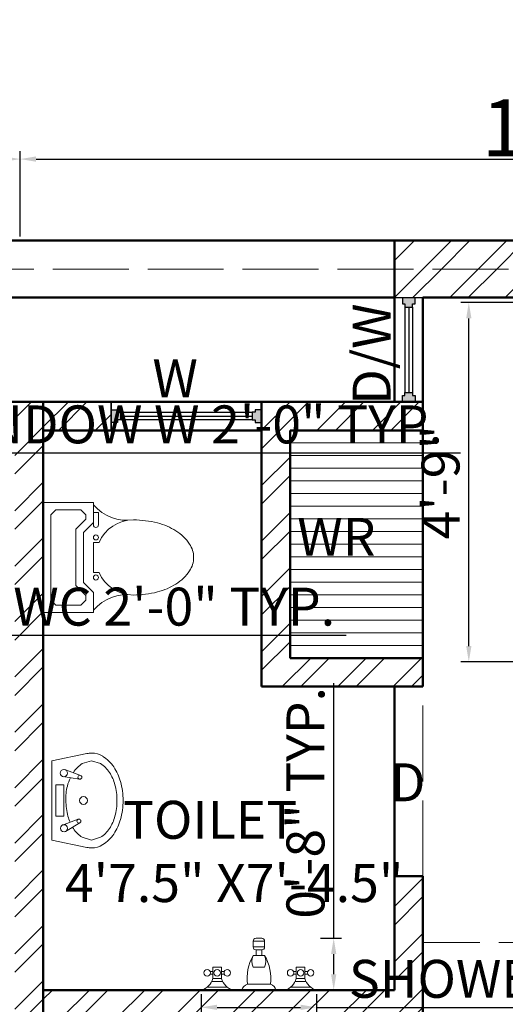
# Model space of a CAD drawing. Units: millimetres. Extents: x 4237 to 5109, y 21391 to 22486.
# Tile 11 of 17: x 4458 to 4535, y 22320 to 22476. Entities that reach past the tile are written whole.
import ezdxf

# ---------------------------------------------------------------- set-up
doc = ezdxf.new("R2010")
doc.units = ezdxf.units.MM
doc.linetypes.add('ACAD_ISO02W100', pattern=[15, 12, -3])
for name, color, linetype, lineweight in [('A-ANNO-DIMS', 2, 'Continuous', 18), ('A-ANNO-TEXT', 7, 'Continuous', 18), ('A-AREA-IDEN', 3, 'Continuous', 18), ('A-FLOR-OVHD', 1, 'ACAD_ISO02W100', 18), ('A-FURN', 8, 'Continuous', 18), ('A-FURN-CASE', 31, 'Continuous', 13), ('A-WALL', 7, 'Continuous', 50), ('A-WALL-PATT', 252, 'Continuous', 13), ('windows', 140, 'Continuous', 25)]:
    doc.layers.add(name, color=color, linetype=linetype, lineweight=lineweight)
doc.styles.get("Standard").update_dxf_attribs({"font": 'arial.ttf'})
doc.dimstyles.new('ISO-25', dxfattribs={"dimtxt": 6, "dimasz": 2.5, "dimexe": 1.25, "dimexo": 0.625, "dimtad": 1, "dimdec": 1, "dimlunit": 4, "dimtxsty": 'Standard', "dimcen": 2.5, "dimadec": 0, "dimazin": 0, "dimtfac": 1, "dimtdec": 1, "dimtmove": 0, "dimatfit": 3, "dimfxl": 1, "dimarcsym": 0})

# ---------------------------------------------------------------- blocks, each defined once
blk = doc.blocks.new('A$C5EF6120A')
at = {"linetype": 'ByBlock'}
for p, q in [((0, 0.762), (0, 0.508)), ((0, 0.762), (0.5588, 0.762)), ((0.5588, 0.762), (0.5588, 0.508)), ((0.0381, 0.6985), (0.0635, 0.7239)), ((0.0635, 0.7239), (0.4953, 0.7239)), ((0.4953, 0.7239), (0.5207, 0.6985)), ((0.0381, 0.6985), (0.0381, 0.5715)), ((0.5207, 0.6985), (0.5207, 0.5715)), ((0.0635, 0.5461), (0.0381, 0.5715)), ((0.1366, 0.5969), (0.0858, 0.5461)), ((0.1524, 0.5588), (0.1016, 0.508)), ((0.1366, 0.5969), (0.4222, 0.5969)), ((0.1524, 0.5588), (0.4064, 0.5588)), ((0.4064, 0.5588), (0.4572, 0.508)), ((0.4222, 0.5969), (0.473, 0.5461)), ((0.5207, 0.5715), (0.4953, 0.5461)), ((0, 0.508), (0.1016, 0.508)), ((0.0508, 0.508), (0.0508, 0.4826)), ((0.0635, 0.5461), (0.0858, 0.5461)), ((0.1143, 0.508), (0.1016, 0.508)), ((0.2032, 0.508), (0.2032, 0.4794)), ((0.3556, 0.508), (0.2032, 0.508)), ((0.3556, 0.508), (0.3556, 0.4794)), ((0.5588, 0.508), (0.4572, 0.508)), ((0.4953, 0.5461), (0.473, 0.5461)), ((0.0508, 0.4826), (0.1143, 0.4826))]:
    blk.add_line(p, q, dxfattribs=at)
blk.add_lwpolyline([(0.0889, 0.3048, 0.063415), (0.1044, 0.183, 0.076468), (0.1447, 0.0893, 0.107136), (0.2118, 0.0204, 0.147373), (0.2794, 0, 0.147373), (0.347, 0.0204, 0.107136), (0.4141, 0.0893, 0.076468), (0.4544, 0.183, 0.063415), (0.4699, 0.3048, 0.063415)], format="xyb", dxfattribs=at)
for centre in [(0.1778, 0.4953), (0.381, 0.4953)]:
    blk.add_circle(centre, 0.0127, dxfattribs=at)
for centre, radius, start, end in [((-0.1375, 0.3358), 0.2285, 352.2011, 48.911), ((0.1143, 0.4953), 0.0127, 270, 90), ((0.6963, 0.3358), 0.2285, 131.089, 187.7989), ((0.2794, 0.3048), 0.1905, 113.5782, 180), ((0.2794, 0.3048), 0.1905, 0, 66.4218)]:
    blk.add_arc(centre, radius, start, end, dxfattribs=at)
blk = doc.blocks.new('A$C60F95712')
for p, q in [((0.05, 0.45), (0.003, 0.2283)), ((0.55, 0.45), (0.05, 0.45)), ((0.597, 0.2283), (0.55, 0.45)), ((0.1448, 0.3831), (0.1814, 0.2836)), ((0.4, 0.425), (0.2, 0.425)), ((0.2, 0.425), (0.2, 0.375)), ((0.2, 0.375), (0.4, 0.375)), ((0.4, 0.375), (0.4, 0.425)), ((0.4514, 0.3804), (0.4348, 0.2751)), ((0.1035, 0.3639), (0.1588, 0.2727)), ((0.4953, 0.3684), (0.459, 0.2688))]:
    blk.add_line(p, q)
for points in [[(0.1307, 0.319, 0.008163), (0.1232, 0.3143, 0.107176), (0.0669, 0.2578), (0.05, 0.2), (0.0669, 0.1422, 0.107176), (0.1232, 0.0857, 0.078233), (0.2003, 0.0515, 0.065516), (0.3, 0.0383, 0.065516), (0.3997, 0.0515, 0.078233), (0.4768, 0.0857, 0.107176), (0.5331, 0.1422), (0.55, 0.2)], [(0.4439, 0.3328, 0.046779), (0.3911, 0.3524, 0.080145), (0.3, 0.3617, 0.065516), (0.2003, 0.3485, 0.037125), (0.1623, 0.3353, 0.107176)], [(0.55, 0.2), (0.5331, 0.2578, 0.107176), (0.4768, 0.3143, 0.000976), (0.4758, 0.3149, 0.080145)]]:
    blk.add_lwpolyline(points, format="xyb")
for centre, radius in [((0.1241, 0.3735), 0.0228), ((0.4733, 0.3744), 0.0228), ((0.1696, 0.2793), 0.0126), ((0.3, 0.25), 0.025), ((0.4472, 0.2731), 0.0126)]:
    blk.add_circle(centre, radius)
for centre, radius, start, end in [((0.1362, 0.2), 0.1362, 168.02396, 180), ((0.1362, 0.2), 0.1362, 180, 211.85353), ((0.4638, 0.2), 0.1362, 328.14647, 0), ((0.4638, 0.2), 0.1362, 0, 11.97604), ((0.2147, 0.2488), 0.2286, 211.85353, 236.30993), ((0.3853, 0.2488), 0.2286, 303.69007, 328.14647), ((0.2662, 0.3261), 0.3215, 236.30993, 254.56292), ((0.3, 0.4484), 0.4484, 254.56292, 270), ((0.3, 0.4484), 0.4484, 270, 285.43708), ((0.3338, 0.3261), 0.3215, 285.43708, 303.69007)]:
    blk.add_arc(centre, radius, start, end)
blk = doc.blocks.new('Faucet - Bathroom front')
for p, q in [((-0.5, 4.25), (0.5, 4.25)), ((0.5, 3.75), (-0.5, 3.75)), ((-0.25, 3), (-0.25, 3.5)), ((0.25, 3.5), (0.25, 3)), ((-0.5, 3), (0.5, 3)), ((0.5, 2), (-0.5, 2)), ((-4, 1.625), (-4.25, 1.625)), ((-4, 1.375), (-4.25, 1.375)), ((-3.25, 1.625), (-3, 1.625)), ((-3.25, 1.375), (-3, 1.375)), ((3.25, 1.625), (3, 1.625)), ((3.25, 1.375), (3, 1.375)), ((4, 1.625), (4.25, 1.625)), ((4, 1.375), (4.25, 1.375)), ((-5, 0), (-2.25, 0)), ((-4.5087, 0.25), (-2.7408, 0.25)), ((-3.1442, 0.75), (-4.0979, 0.75)), ((-1.5, 0), (1.5, 0)), ((-1, 0.5), (1, 0.5)), ((2.25, 0), (5, 0)), ((2.7413, 0.25), (4.5092, 0.25)), ((4.1058, 0.75), (3.1521, 0.75))]:
    blk.add_line(p, q)
for points in [[(-0.25, 4.5), (0.25, 4.5)], [(-0.5, 3.75), (-0.5, 4.25)], [(0.25, 3.5), (-0.25, 3.5)], [(0.5, 4.25), (0.5, 3.75)]]:
    blk.add_lwpolyline(points)
for points in [[(-4, 1), (-4, 2), (-3.25, 2), (-3.25, 1)], [(3.25, 1), (3.25, 2), (4, 2), (4, 1)]]:
    blk.add_lwpolyline(points, close=True)
for centre in [(-4.5, 1.5), (-3.625, 1.5), (-2.75, 1.5), (2.75, 1.5), (3.625, 1.5), (4.5, 1.5)]:
    blk.add_circle(centre, 0.2795)
for centre, radius, start, end in [((-0.2575, 4.2575), 0.2426, 88.22243, 181.7776), ((0.2575, 4.2575), 0.2426, 358.2224, 91.77757), ((-0.2575, 3.7425), 0.2426, 178.2224, 271.7776), ((0.2575, 3.7425), 0.2426, 268.2224, 1.777565), ((3, 1), 4.0311, 150.2551, 187.125), ((0.6413, 2.5), 1.246, 156.3417, 203.6583), ((-3, 1), 4.0311, 352.875, 29.74488), ((-0.6413, 2.5), 1.246, 336.3417, 23.65835), ((-5.375, 1.375), 1.4252, 285.2551, 344.7449), ((-1.875, 1.375), 1.4252, 195.2551, 254.7449), ((1.875, 1.375), 1.4252, 285.2551, 344.7449), ((5.375, 1.375), 1.4252, 195.2551, 254.7449), ((-0.7962, -0.2038), 0.7327, 106.1502, 163.8498), ((0.7962, -0.2038), 0.7327, 16.1502, 73.84979)]:
    blk.add_arc(centre, radius, start, end)
blk = doc.blocks.new('*D56')
at = {"layer": 'A-ANNO-DIMS', "color": 0, "lineweight": -2, "transparency": 16777216}
for p, q in [((4271.65, 22441.33), (4271.65, 22454.84)), ((4274.15, 22453.59), (4455.8, 22453.59)), ((4458.3, 22441.33), (4458.3, 22454.84))]:
    blk.add_line(p, q, dxfattribs=at)
at = {"layer": 'A-ANNO-DIMS', "color": 0, "transparency": 16777216}
for points in [[(4274.15, 22454.01), (4274.15, 22453.17), (4271.65, 22453.59)], [(4455.8, 22454.01), (4455.8, 22453.17), (4458.3, 22453.59)]]:
    blk.add_solid(points, dxfattribs=at)
at = {"layer": 'Defpoints', "color": 0, "transparency": 16777216}
for p in [(4458.3, 22453.59), (4271.65, 22440.7), (4458.3, 22440.7)]:
    blk.add_point(p, dxfattribs=at)
at = {"layer": 'A-ANNO-DIMS', "color": 0, "transparency": 16777216, "insert": (4364.98, 22464.83), "char_height": 9, "attachment_point": 5}
blk.add_mtext('15\'-6{\\H1x;\\S1/2;}"', dxfattribs=at)
blk = doc.blocks.new('*D57')
at = {"layer": 'A-ANNO-DIMS', "color": 0, "lineweight": -2, "transparency": 16777216}
for p, q in [((4458.3, 22441.33), (4458.3, 22454.84)), ((4460.8, 22453.59), (4642.45, 22453.59)), ((4644.95, 22441.33), (4644.95, 22454.84))]:
    blk.add_line(p, q, dxfattribs=at)
at = {"layer": 'A-ANNO-DIMS', "color": 0, "transparency": 16777216}
for points in [[(4460.8, 22454.01), (4460.8, 22453.17), (4458.3, 22453.59)], [(4642.45, 22454.01), (4642.45, 22453.17), (4644.95, 22453.59)]]:
    blk.add_solid(points, dxfattribs=at)
at = {"layer": 'Defpoints', "color": 0, "transparency": 16777216}
for p in [(4644.95, 22453.59), (4458.3, 22440.7), (4644.95, 22440.7)]:
    blk.add_point(p, dxfattribs=at)
at = {"layer": 'A-ANNO-DIMS', "color": 0, "transparency": 16777216, "insert": (4551.63, 22464.83), "char_height": 9, "attachment_point": 5}
blk.add_mtext('15\'-6{\\H1x;\\S1/2;}"', dxfattribs=at)
blk = doc.blocks.new('WIN-A')
blk.add_line((0, 4.5), (0, 0))
blk.add_lwpolyline([(0, 4.5), (23.8, 4.5), (23.8, 0), (0, 0)], close=True)
blk = doc.blocks.new('*D67')
at = {"layer": 'A-ANNO-DIMS', "color": 0, "lineweight": -2, "transparency": 16777216}
for p, q in [((4540.51, 22430.91), (4527.94, 22430.91)), ((4529.19, 22376.6), (4529.19, 22428.41)), ((4540.51, 22374.1), (4527.94, 22374.1))]:
    blk.add_line(p, q, dxfattribs=at)
at = {"layer": 'A-ANNO-DIMS', "color": 0, "transparency": 16777216}
for points in [[(4528.78, 22428.41), (4529.61, 22428.41), (4529.19, 22430.91)], [(4528.78, 22376.6), (4529.61, 22376.6), (4529.19, 22374.1)]]:
    blk.add_solid(points, dxfattribs=at)
at = {"layer": 'Defpoints', "color": 0, "transparency": 16777216}
for p in [(4529.19, 22430.91), (4541.13, 22430.91), (4541.13, 22374.1)]:
    blk.add_point(p, dxfattribs=at)
at = {"layer": 'A-ANNO-DIMS', "color": 0, "transparency": 16777216, "insert": (4525.5, 22402.5), "char_height": 6, "attachment_point": 5, "rotation": 90}
blk.add_mtext('4\'-9"', dxfattribs=at)
blk = doc.blocks.new('*D76')
at = {"layer": 'A-ANNO-DIMS', "color": 0, "lineweight": -2, "transparency": 16777216}
for p, q in [((4429.2, 22381.26), (4429.2, 22377.08)), ((4452.95, 22381.26), (4452.95, 22377.08)), ((4431.7, 22378.33), (4450.45, 22378.33)), ((4452.95, 22378.33), (4509.81, 22378.33))]:
    blk.add_line(p, q, dxfattribs=at)
at = {"layer": 'A-ANNO-DIMS', "color": 0, "transparency": 16777216}
for points in [[(4431.7, 22378.74), (4431.7, 22377.91), (4429.2, 22378.33)], [(4450.45, 22378.74), (4450.45, 22377.91), (4452.95, 22378.33)]]:
    blk.add_solid(points, dxfattribs=at)
at = {"layer": 'Defpoints', "color": 0, "transparency": 16777216}
for p in [(4429.2, 22381.89), (4452.95, 22381.89), (4452.95, 22378.33)]:
    blk.add_point(p, dxfattribs=at)
at = {"layer": 'A-ANNO-DIMS', "color": 0, "transparency": 16777216, "insert": (4482.63, 22382.05), "char_height": 6, "attachment_point": 5}
blk.add_mtext('WC 2\'-0" TYP.', dxfattribs=at)
blk = doc.blocks.new('*D80')
at = {"layer": 'A-ANNO-DIMS', "color": 0, "lineweight": -2, "transparency": 16777216}
for p, q in [((4414.15, 22410.08), (4414.15, 22405.88)), ((4437.95, 22410.08), (4437.95, 22405.88)), ((4416.65, 22407.13), (4435.45, 22407.13)), ((4437.95, 22407.13), (4527.87, 22407.13))]:
    blk.add_line(p, q, dxfattribs=at)
at = {"layer": 'A-ANNO-DIMS', "color": 0, "transparency": 16777216}
for points in [[(4416.65, 22407.55), (4416.65, 22406.71), (4414.15, 22407.13)], [(4435.45, 22407.55), (4435.45, 22406.71), (4437.95, 22407.13)]]:
    blk.add_solid(points, dxfattribs=at)
at = {"layer": 'Defpoints', "color": 0, "transparency": 16777216}
for p in [(4414.15, 22410.7), (4437.95, 22410.7), (4437.95, 22407.13)]:
    blk.add_point(p, dxfattribs=at)
at = {"layer": 'A-ANNO-DIMS', "color": 0, "transparency": 16777216, "insert": (4484.16, 22410.86), "char_height": 6, "attachment_point": 5}
blk.add_mtext('WINDOW W 2\'-0" TYP.', dxfattribs=at)
blk = doc.blocks.new('*D90')
at = {"layer": 'A-ANNO-DIMS', "color": 0, "lineweight": -2, "transparency": 16777216}
for p, q in [((4486.92, 22321.58), (4486.92, 22318.22)), ((4505.11, 22321.58), (4505.11, 22318.22)), ((4489.42, 22319.47), (4502.61, 22319.47)), ((4505.11, 22319.47), (4585.45, 22319.47))]:
    blk.add_line(p, q, dxfattribs=at)
at = {"layer": 'A-ANNO-DIMS', "color": 0, "transparency": 16777216}
for points in [[(4489.42, 22319.89), (4489.42, 22319.06), (4486.92, 22319.47)], [(4502.61, 22319.89), (4502.61, 22319.06), (4505.11, 22319.47)]]:
    blk.add_solid(points, dxfattribs=at)
at = {"layer": 'Defpoints', "color": 0, "transparency": 16777216}
for p in [(4486.92, 22322.2), (4505.11, 22322.2), (4505.11, 22319.47)]:
    blk.add_point(p, dxfattribs=at)
at = {"layer": 'A-ANNO-DIMS', "color": 0, "transparency": 16777216, "insert": (4546.53, 22323.2), "char_height": 6, "attachment_point": 5}
blk.add_mtext('SHOWER 1\'-6" TYP.', dxfattribs=at)
blk = doc.blocks.new('*D91')
at = {"layer": 'A-ANNO-DIMS', "color": 0, "lineweight": -2, "transparency": 16777216}
for p, q in [((4507.84, 22330.39), (4507.84, 22370.71)), ((4505.74, 22330.39), (4509.09, 22330.39)), ((4507.84, 22324.7), (4507.84, 22327.89)), ((4505.74, 22322.2), (4509.09, 22322.2))]:
    blk.add_line(p, q, dxfattribs=at)
at = {"layer": 'A-ANNO-DIMS', "color": 0, "transparency": 16777216}
for points in [[(4507.42, 22327.89), (4508.26, 22327.89), (4507.84, 22330.39)], [(4507.42, 22324.7), (4508.26, 22324.7), (4507.84, 22322.2)]]:
    blk.add_solid(points, dxfattribs=at)
at = {"layer": 'Defpoints', "color": 0, "transparency": 16777216}
for p in [(4505.11, 22330.39), (4507.84, 22330.39), (4505.11, 22322.2)]:
    blk.add_point(p, dxfattribs=at)
at = {"layer": 'A-ANNO-DIMS', "color": 0, "transparency": 16777216, "insert": (4504.15, 22351.8), "char_height": 6, "attachment_point": 5, "rotation": 90}
blk.add_mtext('0\'-8" TYP.', dxfattribs=at)

msp = doc.modelspace()

# ---------------------------------------------------------------- hatches: boundary and pattern name
at = {"layer": 'A-WALL-PATT'}
h = msp.add_hatch(dxfattribs=at)
h.set_pattern_fill('ANSI32', color=256, scale=0.65)
h.paths.add_polyline_path([(4644.95, 22440.7), (4517.45, 22440.7), (4517.45, 22436.2), (4622.45, 22436.2), (4640.45, 22436.2), (4640.45, 22427.2), (4640.45, 22233.7), (4644.95, 22233.7)])
h = msp.add_hatch(dxfattribs=at)
h.set_pattern_fill('ANSI32', color=256, scale=0.65)
h.paths.add_polyline_path([(4622.45, 22436.2), (4517.45, 22436.2), (4517.45, 22431.7), (4521.95, 22431.7), (4622.45, 22431.7)], flags=17)
h = msp.add_hatch(color=256, dxfattribs=at)
h.dxf.hatch_style = 1
h.paths.add_polyline_path([(4520.7, 22431.7), (4518.7, 22431.7), (4518.7, 22430.7), (4519.09, 22430.7), (4519.09, 22430.19), (4520.31, 22430.19), (4520.31, 22430.7), (4520.7, 22430.7)])
h = msp.add_hatch(color=256, dxfattribs=at)
h.dxf.hatch_style = 1
h.paths.add_polyline_path([(4520.7, 22416.2), (4520.31, 22416.2), (4520.31, 22416.71), (4519.09, 22416.71), (4519.09, 22416.2), (4518.7, 22416.2), (4518.7, 22415.2), (4520.7, 22415.2)])
h = msp.add_hatch(dxfattribs=at)
h.set_pattern_fill('ANSI32', color=256, scale=0.65)
h.paths.add_polyline_path([(4461.95, 22415.2), (4457.45, 22415.2), (4457.45, 22233.7), (4461.95, 22233.7)])
h = msp.add_hatch(dxfattribs=at)
h.set_pattern_fill('ANSI32', color=256, scale=0.65)
h.paths.add_polyline_path([(4472.65, 22415.2), (4461.95, 22415.2), (4461.95, 22410.7), (4472.65, 22410.7)])
h = msp.add_hatch(dxfattribs=at)
h.set_pattern_fill('ANSI32', color=256, scale=0.65)
h.paths.add_polyline_path([(4521.95, 22415.2), (4517.45, 22415.2), (4496.45, 22415.2), (4496.45, 22410.7), (4496.45, 22370.2), (4521.95, 22370.2), (4521.95, 22374.7), (4500.95, 22374.7), (4500.95, 22410.7), (4521.95, 22410.7)])
h = msp.add_hatch(color=256, dxfattribs=at)
h.dxf.hatch_style = 1
h.paths.add_polyline_path([(4474.17, 22413.56), (4473.65, 22413.56), (4473.65, 22413.95), (4472.65, 22413.95), (4472.65, 22411.95), (4473.65, 22411.95), (4473.65, 22412.34), (4474.17, 22412.34)])
h = msp.add_hatch(color=256, dxfattribs=at)
h.dxf.hatch_style = 1
h.paths.add_polyline_path([(4496.45, 22413.95), (4495.45, 22413.95), (4495.45, 22413.56), (4494.94, 22413.56), (4494.94, 22412.34), (4495.45, 22412.34), (4495.45, 22411.95), (4496.45, 22411.95)])
h = msp.add_hatch(dxfattribs=at)
h.set_pattern_fill('ANSI32', color=256, scale=0.65)
h.paths.add_polyline_path([(4521.95, 22340.2), (4517.45, 22340.2), (4517.45, 22322.2), (4461.95, 22322.2), (4461.95, 22317.7), (4521.95, 22317.7)])

# ---------------------------------------------------------------- linework, layer by layer
at = {"layer": 'A-FLOR-OVHD'}
for p, q in [((4521.95, 22340.2), (4521.95, 22370.2)), ((4560.95, 22329.7), (4521.95, 22329.7))]:
    msp.add_line(p, q, dxfattribs=at)
msp.add_lwpolyline([(4640.45, 22032.7), (4640.45, 22436.2), (4276.15, 22436.2), (4276.15, 22032.7)], dxfattribs=at)
at = {"layer": 'A-FURN-CASE'}
for p, q in [((4500.95, 22408.7), (4521.95, 22408.7)), ((4500.95, 22406.7), (4521.95, 22406.7)), ((4500.95, 22404.7), (4521.95, 22404.7)), ((4500.95, 22402.7), (4521.95, 22402.7)), ((4500.95, 22400.7), (4521.95, 22400.7)), ((4500.95, 22398.7), (4521.95, 22398.7)), ((4500.95, 22396.7), (4521.95, 22396.7)), ((4500.95, 22394.7), (4521.95, 22394.7)), ((4500.95, 22392.7), (4521.95, 22392.7)), ((4500.95, 22390.7), (4521.95, 22390.7)), ((4500.95, 22388.7), (4521.95, 22388.7)), ((4500.95, 22386.7), (4521.95, 22386.7)), ((4500.95, 22384.7), (4521.95, 22384.7)), ((4500.95, 22382.7), (4521.95, 22382.7)), ((4500.95, 22380.7), (4521.95, 22380.7)), ((4500.95, 22378.7), (4521.95, 22378.7)), ((4500.95, 22376.7), (4521.95, 22376.7))]:
    msp.add_line(p, q, dxfattribs=at)
at = {"layer": 'A-WALL'}
for p, q in [((4271.65, 22440.7), (4644.95, 22440.7)), ((4517.45, 22440.7), (4517.45, 22415.2)), ((4399.15, 22431.7), (4517.45, 22431.7)), ((4521.95, 22431.7), (4521.95, 22370.2)), ((4521.95, 22431.7), (4622.45, 22431.7)), ((4394.65, 22415.2), (4521.95, 22415.2)), ((4461.95, 22415.2), (4461.95, 22233.7)), ((4496.45, 22415.2), (4496.45, 22370.2)), ((4496.45, 22415.2), (4496.45, 22410.7)), ((4461.95, 22410.7), (4496.45, 22410.7)), ((4500.95, 22410.7), (4500.95, 22374.7)), ((4500.95, 22410.7), (4521.95, 22410.7)), ((4500.95, 22374.7), (4521.95, 22374.7)), ((4496.45, 22370.2), (4521.95, 22370.2)), ((4517.45, 22340.2), (4517.45, 22370.2)), ((4517.45, 22340.2), (4517.45, 22322.2)), ((4517.45, 22340.2), (4521.95, 22340.2)), ((4521.95, 22340.2), (4521.95, 22317.7)), ((4461.95, 22322.2), (4517.45, 22322.2))]:
    msp.add_line(p, q, dxfattribs=at)
at = {"layer": 'windows'}
for p, q in [((4519.09, 22430.19), (4519.09, 22416.71)), ((4519.7, 22430.19), (4519.7, 22416.71)), ((4520.31, 22430.19), (4520.31, 22416.71)), ((4474.17, 22413.56), (4494.94, 22413.56)), ((4474.17, 22412.95), (4494.94, 22412.95)), ((4494.94, 22412.34), (4474.17, 22412.34))]:
    msp.add_line(p, q, dxfattribs=at)
msp.add_lwpolyline([(4517.45, 22431.7), (4521.95, 22431.7), (4521.95, 22415.2), (4517.45, 22415.2)], close=True, dxfattribs=at)
for points in [[(4518.7, 22431.7), (4518.7, 22430.7), (4519.09, 22430.7), (4519.09, 22430.19), (4520.31, 22430.19), (4520.31, 22430.7), (4520.7, 22430.7), (4520.7, 22431.7)], [(4518.7, 22415.2), (4518.7, 22416.2), (4519.09, 22416.2), (4519.09, 22416.71), (4520.31, 22416.71), (4520.31, 22416.2), (4520.7, 22416.2), (4520.7, 22415.2)], [(4472.65, 22413.95), (4473.65, 22413.95), (4473.65, 22413.56), (4474.17, 22413.56), (4474.17, 22412.34), (4473.65, 22412.34), (4473.65, 22411.95), (4472.65, 22411.95)], [(4496.45, 22413.95), (4495.45, 22413.95), (4495.45, 22413.56), (4494.94, 22413.56), (4494.94, 22412.34), (4495.45, 22412.34), (4495.45, 22411.95), (4496.45, 22411.95)]]:
    msp.add_lwpolyline(points, dxfattribs=at)

# ---------------------------------------------------------------- block references
at = {"layer": 'A-FURN', "rotation": 90}
for name, p, xscale, yscale, zscale in [('A$C5EF6120A', (4485.7, 22399.31), -31.17096342775826, 31.17096342775826, 31.17096342775826), ('A$C60F95712', (4474.55, 22344.68), 24.9845081568618, 24.9845081568618, 24.9845081568618)]:
    msp.add_blockref(name, p, dxfattribs=dict(at, xscale=xscale, yscale=yscale, zscale=zscale))
at = {"layer": 'A-FURN', "xscale": 1.818895909746216, "yscale": 1.818895909746216, "zscale": 1.818895909746216}
msp.add_blockref('Faucet - Bathroom front', (4496.02, 22322.2), dxfattribs=at)
at = {"layer": 'windows'}
msp.add_blockref('WIN-A', (4472.65, 22410.7), dxfattribs=at)

# ---------------------------------------------------------------- texts
at = {"layer": 'A-ANNO-TEXT', "insert": (4510.83, 22412.91), "char_height": 6, "attachment_point": 1, "rotation": 90}
msp.add_mtext_dynamic_manual_height_columns(' D/W', width=21.7253, gutter_width=12.5, heights=[0], dxfattribs=at)
at = {"layer": 'A-ANNO-TEXT', "char_height": 6, "attachment_point": 1}
for s, insert in [('    W', (4471.86, 22421.93)), ('   WR', (4496.57, 22396.86)), ('    D', (4509.38, 22358.05))]:
    msp.add_mtext_dynamic_manual_height_columns(s, width=21.7253, gutter_width=12.5, heights=[0], dxfattribs=dict(at, insert=insert))
at = {"layer": 'A-AREA-IDEN', "insert": (4465.37, 22352.12), "char_height": 6, "attachment_point": 1}
msp.add_mtext_dynamic_manual_height_columns('     TOILET\\P4\'7.5" X7\'-4.5"', width=55.7646, gutter_width=12.5, heights=[0], dxfattribs=at)

# ---------------------------------------------------------------- dimensions: what is measured, and where the dimension line sits
at = {"layer": 'A-ANNO-DIMS'}
for base, p1, p2, picture, middle in [((4458.30138825, 22453.59015802), (4271.65138825, 22440.70062861), (4458.30138825, 22440.70062861), '*D56', (4364.97638825, 22464.82873237)), ((4644.95138825, 22453.59015802), (4458.30138825, 22440.70062861), (4644.95138825, 22440.70062861), '*D57', (4551.62638825, 22464.82873237))]:
    dim = msp.add_linear_dim(base=base, p1=p1, p2=p2, dimstyle='ISO-25', override={"dimtxt": 9, "dimclrd": 0, "dimclre": 0, "dimclrt": 0}, dxfattribs=at)
    dim.commit()
    dim.dimension.update_dxf_attribs({"geometry": picture, "text_midpoint": middle})
dim = msp.add_linear_dim(base=(4529.19, 22430.91), p1=(4541.13, 22374.1), p2=(4541.13, 22430.91), angle=90, dimstyle='ISO-25', override={"dimdec": 1, "dimrnd": 0, "dimzin": 1, "dimlunit": 4, "dimfrac": 2}, dxfattribs=at)
dim.commit()
dim.dimension.update_dxf_attribs({"geometry": '*D67', "text_midpoint": (4525.5, 22402.5)})
for base, p1, p2, text, picture, middle in [((4437.95, 22407.13), (4414.15, 22410.7), (4437.95, 22410.7), 'WINDOW W <> TYP.', '*D80', (4484.16, 22410.86)), ((4452.9514, 22378.3263), (4429.1991, 22381.8892), (4452.9514, 22381.8892), 'WC <> TYP.', '*D76', (4482.6323, 22382.0536)), ((4505.11, 22319.47), (4486.92, 22322.2), (4505.11, 22322.2), 'SHOWER <> TYP.', '*D90', (4546.53, 22323.2))]:
    dim = msp.add_linear_dim(base=base, p1=p1, p2=p2, text=text, dimstyle='ISO-25', override={"dimdec": 1, "dimrnd": 0, "dimzin": 1, "dimlunit": 4, "dimfrac": 2}, dxfattribs=at)
    dim.commit()
    dim.dimension.update_dxf_attribs({"geometry": picture, "text_midpoint": middle})
dim = msp.add_linear_dim(base=(4507.84, 22330.39), p1=(4505.11, 22322.2), p2=(4505.11, 22330.39), angle=90, text='<> TYP.', dimstyle='ISO-25', override={"dimdec": 1, "dimrnd": 0, "dimzin": 1, "dimlunit": 4, "dimfrac": 2}, dxfattribs=at)
dim.commit()
dim.dimension.update_dxf_attribs({"geometry": '*D91', "text_midpoint": (4504.15, 22351.8)})

doc.saveas('drawing.dxf')
